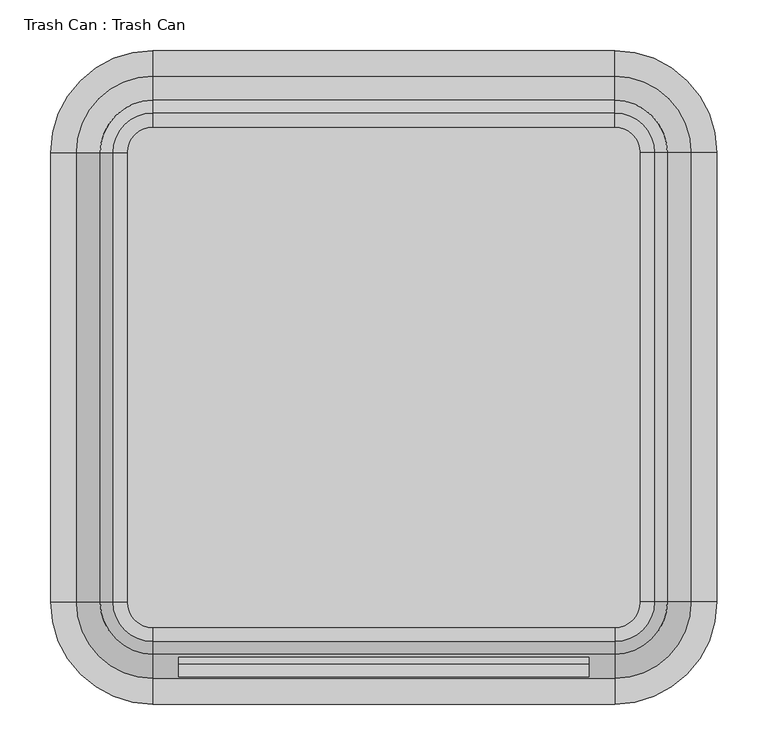
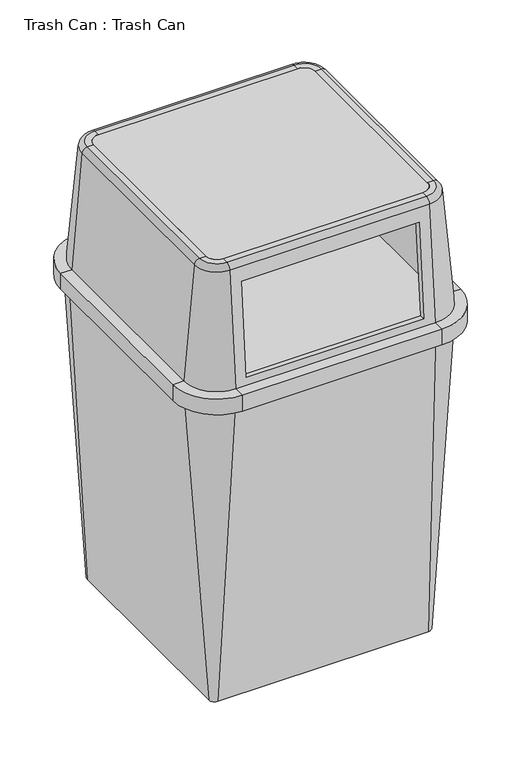
"""IFC4 building model written with IfcOpenShell, lengths in millimetres: geographic element geometry, Trash Can : Trash Can."""

from ifc_helpers import new_model, si_unit, point, frame, frame_2d, origin, place, context, project, spatial, polyline, circle_curve, ellipse_curve, trimmed, segment, composite_curve, outline, extrude, source, transform, mapped, element, save
from ifc_brep_helpers import plane_surface, cylinder_surface, revolved_surface, spline_surface, advanced_brep


def trash_can_trash_can_952d1acd(model_context):
    return source(origin(), model_context, "Body", "SolidModel", [
        advanced_brep(
        [(-254.0, 215.9, 1066.8), (-228.6, 241.3, 1066.8), (-228.6, 255.0625941, 1066.8), (-267.7625941, 215.9, 1066.8), (-254.0, 215.9, 1054.1), (-228.6, 241.3, 1054.1), (-267.7625941, 215.9, 1054.1), (-228.6, 255.0625941, 1054.1), (-292.6673476, 215.9, 769.437365), (-228.6, 279.9673476, 769.437365), (-317.0047535, 215.9, 769.437365), (-228.6, 304.3047535, 769.437365), (-317.0047535, 215.9, 744.037365), (-228.6, 304.3047535, 744.037365), (-329.7047535, 215.9, 744.037365), (-228.6, 317.0047535, 744.037365), (-329.7047535, 215.9, 782.137365), (-228.6, 317.0047535, 782.137365), (-304.3047535, 215.9, 782.137365), (-228.6, 291.6047535, 782.137365), (-280.4142668, 215.9, 1055.2068779), (-228.6, 267.7142668, 1055.2068779), (-267.7625941, -228.6, 1066.8), (-254.0, -228.6, 1066.8), (-254.0, -228.6, 1054.1), (-267.7625941, -228.6, 1054.1), (-292.6673476, -228.6, 769.437365), (-317.0047535, -228.6, 769.437365), (-317.0047535, -228.6, 744.037365), (-329.7047535, -228.6, 744.037365), (-329.7047535, -228.6, 782.137365), (-304.3047535, -228.6, 782.137365), (-280.4142668, -228.6, 1055.2068779), (-228.6, -267.7625941, 1066.8), (-228.6, -254.0, 1066.8), (-228.6, -254.0, 1054.1), (-228.6, -267.7625941, 1054.1), (-228.6, -292.6673476, 769.437365), (-228.6, -317.0047535, 769.437365), (-228.6, -317.0047535, 744.037365), (-228.6, -329.7047535, 744.037365), (-228.6, -329.7047535, 782.137365), (-228.6, -304.3047535, 782.137365), (-228.6, -280.4142668, 1055.2068779), (228.6, -267.7625941, 1066.8), (228.6, -254.0, 1066.8), (228.6, -254.0, 1054.1), (228.6, -267.7625941, 1054.1), (228.6, -292.6673476, 769.437365), (203.2, -290.0863084, 798.9387774), (203.2, -270.7170435, 1020.3304889), (-203.2, -270.7170435, 1020.3304889), (-203.2, -290.0863084, 798.9387774), (228.6, -317.0047535, 769.437365), (228.6, -317.0047535, 744.037365), (228.6, -329.7047535, 744.037365), (228.6, -329.7047535, 782.137365), (228.6, -304.3047535, 782.137365), (228.6, -280.4142668, 1055.2068779), (203.2, -283.3687161, 1021.4373669), (203.2, -302.7379811, 800.0456554), (-203.2, -302.7379811, 800.0456554), (-203.2, -283.3687161, 1021.4373669), (267.7625941, -228.6, 1066.8), (254.0, -228.6, 1066.8), (254.0, -228.6, 1054.1), (267.7625941, -228.6, 1054.1), (292.6673476, -228.6, 769.437365), (317.0047535, -228.6, 769.437365), (317.0047535, -228.6, 744.037365), (329.7047535, -228.6, 744.037365), (329.7047535, -228.6, 782.137365), (304.3047535, -228.6, 782.137365), (280.4142668, -228.6, 1055.2068779), (267.7625941, 215.9, 1066.8), (254.0, 215.9, 1066.8), (254.0, 215.9, 1054.1), (267.7625941, 215.9, 1054.1), (292.6673476, 215.9, 769.437365), (317.0047535, 215.9, 769.437365), (317.0047535, 215.9, 744.037365), (329.7047535, 215.9, 744.037365), (329.7047535, 215.9, 782.137365), (304.3047535, 215.9, 782.137365), (280.4142668, 215.9, 1055.2068779), (228.6, 255.0625941, 1066.8), (228.6, 241.3, 1066.8), (228.6, 241.3, 1054.1), (228.6, 255.0625941, 1054.1), (228.6, 279.9673476, 769.437365), (228.6, 304.3047535, 769.437365), (228.6, 304.3047535, 744.037365), (228.6, 317.0047535, 744.037365), (228.6, 317.0047535, 782.137365), (228.6, 291.6047535, 782.137365), (228.6, 267.7142668, 1055.2068779)],
        [
            (0, 1, circle_curve(frame((-228.6, 215.9, 1066.8), z_axis=(0.0, 0.0, -1.0), x_axis=(0.0, 1.0, 0.0)), 25.4)),
            (1, 2),
            (2, 3, circle_curve(frame((-228.6, 215.9, 1066.8), z_axis=(0.0, 0.0, 1.0), x_axis=(0.0, 1.0, 0.0)), 39.1625941)),
            (3, 0),
            (0, 4),
            (4, 5, circle_curve(frame((-228.6, 215.9, 1054.1), z_axis=(0.0, 0.0, -1.0), x_axis=(0.0, 1.0, 0.0)), 25.4)),
            (5, 1),
            (4, 6),
            (6, 7, circle_curve(frame((-228.6, 215.9, 1054.1), z_axis=(0.0, 0.0, -1.0), x_axis=(0.0, 1.0, 0.0)), 39.1625941)),
            (7, 5),
            (6, 8),
            (8, 9, circle_curve(frame((-228.6, 215.9, 769.437365), z_axis=(0.0, 0.0, -1.0), x_axis=(0.0, 1.0, 0.0)), 64.0673476)),
            (9, 7),
            (8, 10),
            (10, 11, circle_curve(frame((-228.6, 215.9, 769.437365), z_axis=(0.0, 0.0, -1.0), x_axis=(0.0, 1.0, 0.0)), 88.4047535)),
            (11, 9),
            (10, 12),
            (12, 13, circle_curve(frame((-228.6, 215.9, 744.037365), z_axis=(0.0, 0.0, -1.0), x_axis=(0.0, 1.0, 0.0)), 88.4047535)),
            (13, 11),
            (12, 14),
            (14, 15, circle_curve(frame((-228.6, 215.9, 744.037365), z_axis=(0.0, 0.0, -1.0), x_axis=(0.0, 1.0, 0.0)), 101.1047535)),
            (15, 13),
            (14, 16),
            (16, 17, circle_curve(frame((-228.6, 215.9, 782.137365), z_axis=(0.0, 0.0, -1.0), x_axis=(0.0, 1.0, 0.0)), 101.1047535)),
            (17, 15),
            (16, 18),
            (18, 19, circle_curve(frame((-228.6, 215.9, 782.137365), z_axis=(0.0, 0.0, -1.0), x_axis=(0.0, 1.0, 0.0)), 75.7047535)),
            (19, 17),
            (18, 20),
            (20, 21, circle_curve(frame((-228.6, 215.9, 1055.2068779), z_axis=(0.0, 0.0, -1.0), x_axis=(0.0, 1.0, 0.0)), 51.8142668)),
            (21, 19),
            (2, 21, circle_curve(frame((-228.6, 255.0625941, 1054.1), z_axis=(-1.0, 0.0, 0.0), x_axis=(0.0, -1.0, 0.0)), 12.7)),
            (20, 3, circle_curve(frame((-267.7625941, 215.9, 1054.1), z_axis=(0.0, 1.0, 0.0), x_axis=(1.0, 0.0, 0.0)), 12.7)),
            (3, 22),
            (22, 23),
            (23, 0),
            (23, 24),
            (24, 4),
            (24, 25),
            (25, 6),
            (25, 26),
            (26, 8),
            (26, 27),
            (27, 10),
            (27, 28),
            (28, 12),
            (28, 29),
            (29, 14),
            (29, 30),
            (30, 16),
            (30, 31),
            (31, 18),
            (31, 32),
            (32, 20),
            (32, 22, circle_curve(frame((-267.7625941, -228.6, 1054.1), z_axis=(0.0, 1.0, 0.0), x_axis=(1.0, 0.0, 0.0)), 12.7)),
            (22, 33, circle_curve(frame((-228.6, -228.6, 1066.8), z_axis=(0.0, 0.0, 1.0), x_axis=(-1.0, 0.0, 0.0)), 39.1625941)),
            (33, 34),
            (34, 23, circle_curve(frame((-228.6, -228.6, 1066.8), z_axis=(0.0, 0.0, -1.0), x_axis=(-1.0, 0.0, 0.0)), 25.4)),
            (34, 35),
            (35, 24, circle_curve(frame((-228.6, -228.6, 1054.1), z_axis=(0.0, 0.0, -1.0), x_axis=(-1.0, 0.0, 0.0)), 25.4)),
            (35, 36),
            (36, 25, circle_curve(frame((-228.6, -228.6, 1054.1), z_axis=(0.0, 0.0, -1.0), x_axis=(-1.0, 0.0, 0.0)), 39.1625941)),
            (36, 37),
            (37, 26, circle_curve(frame((-228.6, -228.6, 769.437365), z_axis=(0.0, 0.0, -1.0), x_axis=(-1.0, 0.0, 0.0)), 64.0673476)),
            (37, 38),
            (38, 27, circle_curve(frame((-228.6, -228.6, 769.437365), z_axis=(0.0, 0.0, -1.0), x_axis=(-1.0, 0.0, 0.0)), 88.4047535)),
            (38, 39),
            (39, 28, circle_curve(frame((-228.6, -228.6, 744.037365), z_axis=(0.0, 0.0, -1.0), x_axis=(-1.0, 0.0, 0.0)), 88.4047535)),
            (39, 40),
            (40, 29, circle_curve(frame((-228.6, -228.6, 744.037365), z_axis=(0.0, 0.0, -1.0), x_axis=(-1.0, 0.0, 0.0)), 101.1047535)),
            (40, 41),
            (41, 30, circle_curve(frame((-228.6, -228.6, 782.137365), z_axis=(0.0, 0.0, -1.0), x_axis=(-1.0, 0.0, 0.0)), 101.1047535)),
            (41, 42),
            (42, 31, circle_curve(frame((-228.6, -228.6, 782.137365), z_axis=(0.0, 0.0, -1.0), x_axis=(-1.0, 0.0, 0.0)), 75.7047535)),
            (42, 43),
            (43, 32, circle_curve(frame((-228.6, -228.6, 1055.2068779), z_axis=(0.0, 0.0, -1.0), x_axis=(-1.0, 0.0, 0.0)), 51.8142668)),
            (43, 33, circle_curve(frame((-228.6, -267.7625941, 1054.1), z_axis=(-1.0, 0.0, 0.0), x_axis=(0.0, 1.0, 0.0)), 12.7)),
            (33, 44),
            (44, 45),
            (45, 34),
            (45, 46),
            (46, 35),
            (46, 47),
            (47, 36),
            (47, 48),
            (48, 37),
            (49, 50),
            (50, 51),
            (51, 52),
            (52, 49),
            (48, 53),
            (53, 38),
            (53, 54),
            (54, 39),
            (54, 55),
            (55, 40),
            (55, 56),
            (56, 41),
            (56, 57),
            (57, 42),
            (57, 58),
            (58, 43),
            (59, 60),
            (60, 61),
            (61, 62),
            (62, 59),
            (58, 44, circle_curve(frame((228.6, -267.7625941, 1054.1), z_axis=(-1.0, 0.0, 0.0), x_axis=(0.0, 1.0, 0.0)), 12.7)),
            (44, 63, circle_curve(frame((228.6, -228.6, 1066.8), z_axis=(0.0, 0.0, 1.0), x_axis=(0.0, -1.0, 0.0)), 39.1625941)),
            (63, 64),
            (64, 45, circle_curve(frame((228.6, -228.6, 1066.8), z_axis=(0.0, 0.0, -1.0), x_axis=(0.0, -1.0, 0.0)), 25.4)),
            (64, 65),
            (65, 46, circle_curve(frame((228.6, -228.6, 1054.1), z_axis=(0.0, 0.0, -1.0), x_axis=(0.0, -1.0, 0.0)), 25.4)),
            (65, 66),
            (66, 47, circle_curve(frame((228.6, -228.6, 1054.1), z_axis=(0.0, 0.0, -1.0), x_axis=(0.0, -1.0, 0.0)), 39.1625941)),
            (66, 67),
            (67, 48, circle_curve(frame((228.6, -228.6, 769.437365), z_axis=(0.0, 0.0, -1.0), x_axis=(0.0, -1.0, 0.0)), 64.0673476)),
            (67, 68),
            (68, 53, circle_curve(frame((228.6, -228.6, 769.437365), z_axis=(0.0, 0.0, -1.0), x_axis=(0.0, -1.0, 0.0)), 88.4047535)),
            (68, 69),
            (69, 54, circle_curve(frame((228.6, -228.6, 744.037365), z_axis=(0.0, 0.0, -1.0), x_axis=(0.0, -1.0, 0.0)), 88.4047535)),
            (69, 70),
            (70, 55, circle_curve(frame((228.6, -228.6, 744.037365), z_axis=(0.0, 0.0, -1.0), x_axis=(0.0, -1.0, 0.0)), 101.1047535)),
            (70, 71),
            (71, 56, circle_curve(frame((228.6, -228.6, 782.137365), z_axis=(0.0, 0.0, -1.0), x_axis=(0.0, -1.0, 0.0)), 101.1047535)),
            (71, 72),
            (72, 57, circle_curve(frame((228.6, -228.6, 782.137365), z_axis=(0.0, 0.0, -1.0), x_axis=(0.0, -1.0, 0.0)), 75.7047535)),
            (72, 73),
            (73, 58, circle_curve(frame((228.6, -228.6, 1055.2068779), z_axis=(0.0, 0.0, -1.0), x_axis=(0.0, -1.0, 0.0)), 51.8142668)),
            (73, 63, circle_curve(frame((267.7625941, -228.6, 1054.1), z_axis=(0.0, -1.0, 0.0), x_axis=(-1.0, 0.0, 0.0)), 12.7)),
            (63, 74),
            (74, 75),
            (75, 64),
            (75, 76),
            (76, 65),
            (76, 77),
            (77, 66),
            (77, 78),
            (78, 67),
            (78, 79),
            (79, 68),
            (79, 80),
            (80, 69),
            (80, 81),
            (81, 70),
            (81, 82),
            (82, 71),
            (82, 83),
            (83, 72),
            (83, 84),
            (84, 73),
            (84, 74, circle_curve(frame((267.7625941, 215.9, 1054.1), z_axis=(0.0, -1.0, 0.0), x_axis=(-1.0, 0.0, 0.0)), 12.7)),
            (74, 85, circle_curve(frame((228.6, 215.9, 1066.8), z_axis=(0.0, 0.0, 1.0), x_axis=(1.0, 0.0, 0.0)), 39.1625941)),
            (85, 86),
            (86, 75, circle_curve(frame((228.6, 215.9, 1066.8), z_axis=(0.0, 0.0, -1.0), x_axis=(1.0, 0.0, 0.0)), 25.4)),
            (86, 87),
            (87, 76, circle_curve(frame((228.6, 215.9, 1054.1), z_axis=(0.0, 0.0, -1.0), x_axis=(1.0, 0.0, 0.0)), 25.4)),
            (87, 88),
            (88, 77, circle_curve(frame((228.6, 215.9, 1054.1), z_axis=(0.0, 0.0, -1.0), x_axis=(1.0, 0.0, 0.0)), 39.1625941)),
            (88, 89),
            (89, 78, circle_curve(frame((228.6, 215.9, 769.437365), z_axis=(0.0, 0.0, -1.0), x_axis=(1.0, 0.0, 0.0)), 64.0673476)),
            (89, 90),
            (90, 79, circle_curve(frame((228.6, 215.9, 769.437365), z_axis=(0.0, 0.0, -1.0), x_axis=(1.0, 0.0, 0.0)), 88.4047535)),
            (90, 91),
            (91, 80, circle_curve(frame((228.6, 215.9, 744.037365), z_axis=(0.0, 0.0, -1.0), x_axis=(1.0, 0.0, 0.0)), 88.4047535)),
            (91, 92),
            (92, 81, circle_curve(frame((228.6, 215.9, 744.037365), z_axis=(0.0, 0.0, -1.0), x_axis=(1.0, 0.0, 0.0)), 101.1047535)),
            (92, 93),
            (93, 82, circle_curve(frame((228.6, 215.9, 782.137365), z_axis=(0.0, 0.0, -1.0), x_axis=(1.0, 0.0, 0.0)), 101.1047535)),
            (93, 94),
            (94, 83, circle_curve(frame((228.6, 215.9, 782.137365), z_axis=(0.0, 0.0, -1.0), x_axis=(1.0, 0.0, 0.0)), 75.7047535)),
            (94, 95),
            (95, 84, circle_curve(frame((228.6, 215.9, 1055.2068779), z_axis=(0.0, 0.0, -1.0), x_axis=(1.0, 0.0, 0.0)), 51.8142668)),
            (95, 85, circle_curve(frame((228.6, 255.0625941, 1054.1), z_axis=(1.0, 0.0, 0.0), x_axis=(0.0, -1.0, 0.0)), 12.7)),
            (1, 86),
            (85, 2),
            (5, 87),
            (7, 88),
            (9, 89),
            (11, 90),
            (13, 91),
            (15, 92),
            (17, 93),
            (19, 94),
            (21, 95),
            (59, 50),
            (49, 60),
            (52, 61),
            (51, 62),
        ],
        [
            plane_surface(frame((-228.6, 215.9, 1066.8), z_axis=(0.0, 0.0, 1.0), x_axis=(0.0, 1.0, 0.0))),
            revolved_surface(polyline([(-228.6, 241.3, 1066.8), (-228.6, 241.3, 1054.1)]), (-228.6, 215.9, 0.0), (0.0, 0.0, 1.0)),
            plane_surface(frame((-228.6, 215.9, 1054.1), z_axis=(0.0, 0.0, -1.0), x_axis=(0.0, 1.0, 0.0))),
            revolved_surface(polyline([(-228.6, 255.0625941, 1054.1), (-228.6, 279.9673476, 769.437365)]), (-228.6, 215.9, 0.0), (0.0, 0.0, 1.0)),
            plane_surface(frame((-228.6, 215.9, 769.437365), z_axis=(0.0, 0.0, -1.0), x_axis=(0.0, 1.0, 0.0))),
            revolved_surface(polyline([(-228.6, 304.3047535, 769.437365), (-228.6, 304.3047535, 744.037365)]), (-228.6, 215.9, 0.0), (0.0, 0.0, 1.0)),
            plane_surface(frame((-228.6, 215.9, 744.037365), z_axis=(0.0, 0.0, -1.0), x_axis=(0.0, 1.0, 0.0))),
            cylinder_surface(frame((-228.6, 215.9, 0.0), z_axis=(0.0, 0.0, 1.0), x_axis=(0.0, 1.0, 0.0)), 101.1047535),
            plane_surface(frame((-228.6, 215.9, 782.137365), z_axis=(0.0, 0.0, 1.0), x_axis=(0.0, 1.0, 0.0))),
            revolved_surface(polyline([(-228.6, 291.6047535, 782.137365), (-228.6, 267.7142668, 1055.2068779)]), (-228.6, 215.9, 0.0), (0.0, 0.0, 1.0)),
            revolved_surface(trimmed(ellipse_curve(frame((-228.6, 255.0625941, 1054.1), z_axis=(1.0, 0.0, 0.0), x_axis=(0.0, -1.0, 0.0)), 12.7, 12.7), [point((-228.6, 267.7142668, 1055.2068779))], [point((-228.6, 255.0625941, 1066.8))], True, "CARTESIAN"), (-228.6, 215.9, 0.0), (0.0, 0.0, 1.0)),
            plane_surface(frame((-267.7625941, 215.9, 1066.8), z_axis=(0.0, 0.0, 1.0), x_axis=(0.0, -1.0, 0.0))),
            plane_surface(frame((-254.0, 215.9, 1066.8), z_axis=(1.0, 0.0, 0.0), x_axis=(0.0, -1.0, 0.0))),
            plane_surface(frame((-254.0, 215.9, 1054.1), z_axis=(0.0, 0.0, -1.0), x_axis=(0.0, -1.0, 0.0))),
            plane_surface(frame((-267.7625941, 215.9, 1054.1), z_axis=(0.9961946980917451, 0.0, -0.08715574274766279), x_axis=(0.0, -1.0, 0.0))),
            plane_surface(frame((-292.6673476, 215.9, 769.437365), z_axis=(0.0, 0.0, -1.0), x_axis=(0.0, -1.0, 0.0))),
            plane_surface(frame((-317.0047535, 215.9, 769.437365), z_axis=(1.0, 0.0, 0.0), x_axis=(0.0, -1.0, 0.0))),
            plane_surface(frame((-317.0047535, 215.9, 744.037365), z_axis=(0.0, 0.0, -1.0), x_axis=(0.0, -1.0, 0.0))),
            plane_surface(frame((-329.7047535, 215.9, 744.037365), z_axis=(-1.0, 0.0, 0.0), x_axis=(0.0, -1.0, 0.0))),
            plane_surface(frame((-329.7047535, 215.9, 782.137365), z_axis=(0.0, 0.0, 1.0), x_axis=(0.0, -1.0, 0.0))),
            plane_surface(frame((-304.3047535, 215.9, 782.137365), z_axis=(-0.9961946980917452, 0.0, 0.08715574274766147), x_axis=(0.0, -1.0, 0.0))),
            cylinder_surface(frame((-267.7625941, 215.9, 1054.1), z_axis=(0.0, 1.0, 0.0), x_axis=(1.0, 0.0, 0.0)), 12.7),
            plane_surface(frame((-228.6, -228.6, 1066.8), z_axis=(0.0, 0.0, 1.0), x_axis=(-1.0, 0.0, 0.0))),
            revolved_surface(polyline([(-254.0, -228.6, 1066.8), (-254.0, -228.6, 1054.1)]), (-228.6, -228.6, 0.0), (0.0, 0.0, 1.0)),
            plane_surface(frame((-228.6, -228.6, 1054.1), z_axis=(0.0, 0.0, -1.0), x_axis=(-1.0, 0.0, 0.0))),
            revolved_surface(polyline([(-267.7625941, -228.6, 1054.1), (-292.6673476, -228.6, 769.437365)]), (-228.6, -228.6, 0.0), (0.0, 0.0, 1.0)),
            plane_surface(frame((-228.6, -228.6, 769.437365), z_axis=(0.0, 0.0, -1.0), x_axis=(-1.0, 0.0, 0.0))),
            revolved_surface(polyline([(-317.0047535, -228.6, 769.437365), (-317.0047535, -228.6, 744.037365)]), (-228.6, -228.6, 0.0), (0.0, 0.0, 1.0)),
            plane_surface(frame((-228.6, -228.6, 744.037365), z_axis=(0.0, 0.0, -1.0), x_axis=(-1.0, 0.0, 0.0))),
            cylinder_surface(frame((-228.6, -228.6, 0.0), z_axis=(0.0, 0.0, 1.0), x_axis=(-1.0, 0.0, 0.0)), 101.1047535),
            plane_surface(frame((-228.6, -228.6, 782.137365), z_axis=(0.0, 0.0, 1.0), x_axis=(-1.0, 0.0, 0.0))),
            revolved_surface(polyline([(-304.3047535, -228.6, 782.137365), (-280.4142668, -228.6, 1055.2068779)]), (-228.6, -228.6, 0.0), (0.0, 0.0, 1.0)),
            revolved_surface(trimmed(ellipse_curve(frame((-267.7625941, -228.6, 1054.1), z_axis=(0.0, 1.0, 0.0), x_axis=(1.0, 0.0, 0.0)), 12.7, 12.7), [point((-280.4142668, -228.6, 1055.2068779))], [point((-267.7625941, -228.6, 1066.8))], True, "CARTESIAN"), (-228.6, -228.6, 0.0), (0.0, 0.0, 1.0)),
            plane_surface(frame((-228.6, -267.7625941, 1066.8), z_axis=(0.0, 0.0, 1.0), x_axis=(1.0, 0.0, 0.0))),
            plane_surface(frame((-228.6, -254.0, 1066.8), z_axis=(0.0, 1.0, 0.0), x_axis=(1.0, 0.0, 0.0))),
            plane_surface(frame((-228.6, -254.0, 1054.1), z_axis=(0.0, 0.0, -1.0), x_axis=(1.0, 0.0, 0.0))),
            plane_surface(frame((-228.6, -267.7625941, 1054.1), z_axis=(0.0, 0.9961946980917451, -0.08715574274766279), x_axis=(1.0, 0.0, 0.0))),
            plane_surface(frame((-228.6, -292.6673476, 769.437365), z_axis=(0.0, 0.0, -1.0), x_axis=(1.0, 0.0, 0.0))),
            plane_surface(frame((-228.6, -317.0047535, 769.437365), z_axis=(0.0, 1.0, 0.0), x_axis=(1.0, 0.0, 0.0))),
            plane_surface(frame((-228.6, -317.0047535, 744.037365), z_axis=(0.0, 0.0, -1.0), x_axis=(1.0, 0.0, 0.0))),
            plane_surface(frame((-228.6, -329.7047535, 744.037365), z_axis=(0.0, -1.0, 0.0), x_axis=(1.0, 0.0, 0.0))),
            plane_surface(frame((-228.6, -329.7047535, 782.137365), z_axis=(0.0, 0.0, 1.0), x_axis=(1.0, 0.0, 0.0))),
            plane_surface(frame((-228.6, -304.3047535, 782.137365), z_axis=(0.0, -0.9961946980917452, 0.08715574274766147), x_axis=(1.0, 0.0, 0.0))),
            cylinder_surface(frame((-228.6, -267.7625941, 1054.1), z_axis=(-1.0, 0.0, 0.0), x_axis=(0.0, 1.0, 0.0)), 12.7),
            plane_surface(frame((228.6, -228.6, 1066.8), z_axis=(0.0, 0.0, 1.0), x_axis=(0.0, -1.0, 0.0))),
            revolved_surface(polyline([(228.6, -254.0, 1066.8), (228.6, -254.0, 1054.1)]), (228.6, -228.6, 0.0), (0.0, 0.0, 1.0)),
            plane_surface(frame((228.6, -228.6, 1054.1), z_axis=(0.0, 0.0, -1.0), x_axis=(0.0, -1.0, 0.0))),
            revolved_surface(polyline([(228.6, -267.7625941, 1054.1), (228.6, -292.6673476, 769.437365)]), (228.6, -228.6, 0.0), (0.0, 0.0, 1.0)),
            plane_surface(frame((228.6, -228.6, 769.437365), z_axis=(0.0, 0.0, -1.0), x_axis=(0.0, -1.0, 0.0))),
            revolved_surface(polyline([(228.6, -317.0047535, 769.437365), (228.6, -317.0047535, 744.037365)]), (228.6, -228.6, 0.0), (0.0, 0.0, 1.0)),
            plane_surface(frame((228.6, -228.6, 744.037365), z_axis=(0.0, 0.0, -1.0), x_axis=(0.0, -1.0, 0.0))),
            cylinder_surface(frame((228.6, -228.6, 0.0), z_axis=(0.0, 0.0, 1.0), x_axis=(0.0, -1.0, 0.0)), 101.1047535),
            plane_surface(frame((228.6, -228.6, 782.137365), z_axis=(0.0, 0.0, 1.0), x_axis=(0.0, -1.0, 0.0))),
            revolved_surface(polyline([(228.6, -304.3047535, 782.137365), (228.6, -280.4142668, 1055.2068779)]), (228.6, -228.6, 0.0), (0.0, 0.0, 1.0)),
            revolved_surface(trimmed(ellipse_curve(frame((228.6, -267.7625941, 1054.1), z_axis=(-1.0, 0.0, 0.0), x_axis=(0.0, 1.0, 0.0)), 12.7, 12.7), [point((228.6, -280.4142668, 1055.2068779))], [point((228.6, -267.7625941, 1066.8))], True, "CARTESIAN"), (228.6, -228.6, 0.0), (0.0, 0.0, 1.0)),
            plane_surface(frame((267.7625941, -228.6, 1066.8), z_axis=(0.0, 0.0, 1.0), x_axis=(0.0, 1.0, 0.0))),
            plane_surface(frame((254.0, -228.6, 1066.8), z_axis=(-1.0, 0.0, 0.0), x_axis=(0.0, 1.0, 0.0))),
            plane_surface(frame((254.0, -228.6, 1054.1), z_axis=(0.0, 0.0, -1.0), x_axis=(0.0, 1.0, 0.0))),
            plane_surface(frame((267.7625941, -228.6, 1054.1), z_axis=(-0.9961946980917451, 0.0, -0.08715574274766279), x_axis=(0.0, 1.0, 0.0))),
            plane_surface(frame((292.6673476, -228.6, 769.437365), z_axis=(0.0, 0.0, -1.0), x_axis=(0.0, 1.0, 0.0))),
            plane_surface(frame((317.0047535, -228.6, 769.437365), z_axis=(-1.0, 0.0, 0.0), x_axis=(0.0, 1.0, 0.0))),
            plane_surface(frame((317.0047535, -228.6, 744.037365), z_axis=(0.0, 0.0, -1.0), x_axis=(0.0, 1.0, 0.0))),
            plane_surface(frame((329.7047535, -228.6, 744.037365), z_axis=(1.0, 0.0, 0.0), x_axis=(0.0, 1.0, 0.0))),
            plane_surface(frame((329.7047535, -228.6, 782.137365), z_axis=(0.0, 0.0, 1.0), x_axis=(0.0, 1.0, 0.0))),
            plane_surface(frame((304.3047535, -228.6, 782.137365), z_axis=(0.9961946980917452, 0.0, 0.08715574274766147), x_axis=(0.0, 1.0, 0.0))),
            cylinder_surface(frame((267.7625941, -228.6, 1054.1), z_axis=(0.0, -1.0, 0.0), x_axis=(-1.0, 0.0, 0.0)), 12.7),
            plane_surface(frame((228.6, 215.9, 1066.8), z_axis=(0.0, 0.0, 1.0), x_axis=(1.0, 0.0, 0.0))),
            revolved_surface(polyline([(254.0, 215.9, 1066.8), (254.0, 215.9, 1054.1)]), (228.6, 215.9, 0.0), (0.0, 0.0, 1.0)),
            plane_surface(frame((228.6, 215.9, 1054.1), z_axis=(0.0, 0.0, -1.0), x_axis=(1.0, 0.0, 0.0))),
            revolved_surface(polyline([(267.7625941, 215.9, 1054.1), (292.6673476, 215.9, 769.437365)]), (228.6, 215.9, 0.0), (0.0, 0.0, 1.0)),
            plane_surface(frame((228.6, 215.9, 769.437365), z_axis=(0.0, 0.0, -1.0), x_axis=(1.0, 0.0, 0.0))),
            revolved_surface(polyline([(317.0047535, 215.9, 769.437365), (317.0047535, 215.9, 744.037365)]), (228.6, 215.9, 0.0), (0.0, 0.0, 1.0)),
            plane_surface(frame((228.6, 215.9, 744.037365), z_axis=(0.0, 0.0, -1.0), x_axis=(1.0, 0.0, 0.0))),
            cylinder_surface(frame((228.6, 215.9, 0.0), z_axis=(0.0, 0.0, 1.0), x_axis=(1.0, 0.0, 0.0)), 101.1047535),
            plane_surface(frame((228.6, 215.9, 782.137365), z_axis=(0.0, 0.0, 1.0), x_axis=(1.0, 0.0, 0.0))),
            revolved_surface(polyline([(304.3047535, 215.9, 782.137365), (280.4142668, 215.9, 1055.2068779)]), (228.6, 215.9, 0.0), (0.0, 0.0, 1.0)),
            revolved_surface(trimmed(ellipse_curve(frame((267.7625941, 215.9, 1054.1), z_axis=(0.0, -1.0, 0.0), x_axis=(-1.0, 0.0, 0.0)), 12.7, 12.7), [point((280.4142668, 215.9, 1055.2068779))], [point((267.7625941, 215.9, 1066.8))], True, "CARTESIAN"), (228.6, 215.9, 0.0), (0.0, 0.0, 1.0)),
            plane_surface(frame((228.6, 255.0625941, 1066.8), z_axis=(0.0, 0.0, 1.0), x_axis=(-1.0, 0.0, 0.0))),
            plane_surface(frame((228.6, 241.3, 1066.8), z_axis=(0.0, -1.0, 0.0), x_axis=(-1.0, 0.0, 0.0))),
            plane_surface(frame((228.6, 241.3, 1054.1), z_axis=(0.0, 0.0, -1.0), x_axis=(-1.0, 0.0, 0.0))),
            plane_surface(frame((228.6, 255.0625941, 1054.1), z_axis=(0.0, -0.9961946980917451, -0.08715574274766279), x_axis=(-1.0, 0.0, 0.0))),
            plane_surface(frame((228.6, 279.9673476, 769.437365), z_axis=(0.0, 0.0, -1.0), x_axis=(-1.0, 0.0, 0.0))),
            plane_surface(frame((228.6, 304.3047535, 769.437365), z_axis=(0.0, -1.0, 0.0), x_axis=(-1.0, 0.0, 0.0))),
            plane_surface(frame((228.6, 304.3047535, 744.037365), z_axis=(0.0, 0.0, -1.0), x_axis=(-1.0, 0.0, 0.0))),
            plane_surface(frame((228.6, 317.0047535, 744.037365), z_axis=(0.0, 1.0, 0.0), x_axis=(-1.0, 0.0, 0.0))),
            plane_surface(frame((228.6, 317.0047535, 782.137365), z_axis=(0.0, 0.0, 1.0), x_axis=(-1.0, 0.0, 0.0))),
            plane_surface(frame((228.6, 291.6047535, 782.137365), z_axis=(0.0, 0.9961946980917452, 0.08715574274766147), x_axis=(-1.0, 0.0, 0.0))),
            cylinder_surface(frame((228.6, 255.0625941, 1054.1), z_axis=(1.0, 0.0, 0.0), x_axis=(0.0, -1.0, 0.0)), 12.7),
            plane_surface(frame((203.2, -213.4252032, 1015.3181024), z_axis=(-1.0, 0.0, 0.0), x_axis=(0.0, -0.9961946980917452, 0.08715574274766175))),
            plane_surface(frame((203.2, -232.7944681, 793.9263909), z_axis=(0.0, 0.08715574274766175, 0.9961946980917452), x_axis=(0.0, -0.9961946980917452, 0.08715574274766175))),
            plane_surface(frame((-203.2, -232.7944681, 793.9263909), z_axis=(1.0, 0.0, 0.0), x_axis=(0.0, -0.9961946980917452, 0.08715574274766175))),
            plane_surface(frame((-203.2, -213.4252032, 1015.3181024), z_axis=(0.0, -0.08715574274766175, -0.9961946980917452), x_axis=(0.0, -0.9961946980917452, 0.08715574274766175))),
        ],
        [
            (0, [[1, 2, 3, 4]]),
            (1, [[-1, 5, 6, 7]]),
            (2, [[-6, 8, 9, 10]]),
            (3, [[-9, 11, 12, 13]]),
            (4, [[-12, 14, 15, 16]]),
            (5, [[-15, 17, 18, 19]]),
            (6, [[-18, 20, 21, 22]]),
            (7, [[-21, 23, 24, 25]]),
            (8, [[-24, 26, 27, 28]]),
            (9, [[-27, 29, 30, 31]]),
            (10, [[-3, 32, -30, 33]]),
            (11, [[-4, 34, 35, 36]]),
            (12, [[-5, -36, 37, 38]]),
            (13, [[-8, -38, 39, 40]]),
            (14, [[-11, -40, 41, 42]]),
            (15, [[-14, -42, 43, 44]]),
            (16, [[-17, -44, 45, 46]]),
            (17, [[-20, -46, 47, 48]]),
            (18, [[-23, -48, 49, 50]]),
            (19, [[-26, -50, 51, 52]]),
            (20, [[-29, -52, 53, 54]]),
            (21, [[-33, -54, 55, -34]]),
            (22, [[-35, 56, 57, 58]]),
            (23, [[-37, -58, 59, 60]]),
            (24, [[-39, -60, 61, 62]]),
            (25, [[-41, -62, 63, 64]]),
            (26, [[-43, -64, 65, 66]]),
            (27, [[-45, -66, 67, 68]]),
            (28, [[-47, -68, 69, 70]]),
            (29, [[-49, -70, 71, 72]]),
            (30, [[-51, -72, 73, 74]]),
            (31, [[-53, -74, 75, 76]]),
            (32, [[-55, -76, 77, -56]]),
            (33, [[-57, 78, 79, 80]]),
            (34, [[-59, -80, 81, 82]]),
            (35, [[-61, -82, 83, 84]]),
            (36, [[-63, -84, 85, 86], [87, 88, 89, 90]]),
            (37, [[-65, -86, 91, 92]]),
            (38, [[-67, -92, 93, 94]]),
            (39, [[-69, -94, 95, 96]]),
            (40, [[-71, -96, 97, 98]]),
            (41, [[-73, -98, 99, 100]]),
            (42, [[-75, -100, 101, 102], [103, 104, 105, 106]]),
            (43, [[-77, -102, 107, -78]]),
            (44, [[-79, 108, 109, 110]]),
            (45, [[-81, -110, 111, 112]]),
            (46, [[-83, -112, 113, 114]]),
            (47, [[-85, -114, 115, 116]]),
            (48, [[-91, -116, 117, 118]]),
            (49, [[-93, -118, 119, 120]]),
            (50, [[-95, -120, 121, 122]]),
            (51, [[-97, -122, 123, 124]]),
            (52, [[-99, -124, 125, 126]]),
            (53, [[-101, -126, 127, 128]]),
            (54, [[-107, -128, 129, -108]]),
            (55, [[-109, 130, 131, 132]]),
            (56, [[-111, -132, 133, 134]]),
            (57, [[-113, -134, 135, 136]]),
            (58, [[-115, -136, 137, 138]]),
            (59, [[-117, -138, 139, 140]]),
            (60, [[-119, -140, 141, 142]]),
            (61, [[-121, -142, 143, 144]]),
            (62, [[-123, -144, 145, 146]]),
            (63, [[-125, -146, 147, 148]]),
            (64, [[-127, -148, 149, 150]]),
            (65, [[-129, -150, 151, -130]]),
            (66, [[-131, 152, 153, 154]]),
            (67, [[-133, -154, 155, 156]]),
            (68, [[-135, -156, 157, 158]]),
            (69, [[-137, -158, 159, 160]]),
            (70, [[-139, -160, 161, 162]]),
            (71, [[-141, -162, 163, 164]]),
            (72, [[-143, -164, 165, 166]]),
            (73, [[-145, -166, 167, 168]]),
            (74, [[-147, -168, 169, 170]]),
            (75, [[-149, -170, 171, 172]]),
            (76, [[-151, -172, 173, -152]]),
            (77, [[-2, 174, -153, 175]]),
            (78, [[-7, 176, -155, -174]]),
            (79, [[-10, 177, -157, -176]]),
            (80, [[-13, 178, -159, -177]]),
            (81, [[-16, 179, -161, -178]]),
            (82, [[-19, 180, -163, -179]]),
            (83, [[-22, 181, -165, -180]]),
            (84, [[-25, 182, -167, -181]]),
            (85, [[-28, 183, -169, -182]]),
            (86, [[-31, 184, -171, -183]]),
            (87, [[-32, -175, -173, -184]]),
            (88, [[185, -87, 186, -103]]),
            (89, [[-186, -90, 187, -104]]),
            (90, [[-187, -89, 188, -105]]),
            (91, [[-185, -106, -188, -88]]),
        ],
    ),
        extrude(outline(composite_curve([segment(trimmed(circle_curve(frame_2d((241.3, 228.6)), 12.7), [point((241.3, 241.3))], [point((254.0, 228.6))], False, "CARTESIAN"), True, "CONTINUOUS"), segment(polyline([(254.0, 228.6), (254.0, -228.6)]), True, "CONTINUOUS"), segment(trimmed(circle_curve(frame_2d((228.6, -228.6)), 25.4), [point((254.0, -228.6))], [point((228.6, -254.0))], False, "CARTESIAN"), True, "CONTINUOUS"), segment(polyline([(228.6, -254.0), (-228.6, -254.0)]), True, "CONTINUOUS"), segment(trimmed(circle_curve(frame_2d((-228.6, -228.6)), 25.4), [point((-228.6, -254.0))], [point((-254.0, -228.6))], False, "CARTESIAN"), True, "CONTINUOUS"), segment(polyline([(-254.0, -228.6), (-254.0, 215.9)]), True, "CONTINUOUS"), segment(trimmed(circle_curve(frame_2d((-228.6, 215.9)), 25.4), [point((-254.0, 215.9))], [point((-228.6, 241.3))], False, "CARTESIAN"), True, "CONTINUOUS"), segment(polyline([(-228.6, 241.3), (241.3, 241.3)]), True, "CONTINUOUS")], self_intersect=False)), frame((0.0, 0.0, 1054.1), z_axis=(0.0, 0.0, 1.0), x_axis=(1.0, 0.0, 0.0)), (0.0, 0.0, 1.0), 12.7),
        advanced_brep(
        [(228.6, 304.8, 762.0), (-228.6, 304.8, 762.0), (-304.8, 228.6, 762.0), (-304.8, -228.6, 762.0), (-228.6, -304.8, 762.0), (228.6, -304.8, 762.0), (304.8, -228.6, 762.0), (304.8, 228.6, 762.0), (241.3, 254.0, 0.0), (254.0, 241.3, 0.0), (254.0, -241.3, 0.0), (241.3, -254.0, 0.0), (-241.3, -254.0, 0.0), (-254.0, -241.3, 0.0), (-254.0, 241.3, 0.0), (-241.3, 254.0, 0.0)],
        [
            (0, 1),
            (1, 2, circle_curve(frame((-228.6, 228.6, 762.0), z_axis=(0.0, 0.0, 1.0), x_axis=(1.0, 0.0, 0.0)), 76.2)),
            (2, 3),
            (3, 4, circle_curve(frame((-228.6, -228.6, 762.0), z_axis=(0.0, 0.0, 1.0), x_axis=(1.0, 0.0, 0.0)), 76.2)),
            (4, 5),
            (5, 6, circle_curve(frame((228.6, -228.6, 762.0), z_axis=(0.0, 0.0, 1.0), x_axis=(1.0, 0.0, 0.0)), 76.2)),
            (6, 7),
            (7, 0, circle_curve(frame((228.6, 228.6, 762.0), z_axis=(0.0, 0.0, 1.0), x_axis=(1.0, 0.0, 0.0)), 76.2)),
            (8, 9, circle_curve(frame((241.3, 241.3, 0.0), z_axis=(0.0, 0.0, -1.0), x_axis=(1.0, 0.0, 0.0)), 12.7)),
            (9, 10),
            (10, 11, circle_curve(frame((241.3, -241.3, 0.0), z_axis=(0.0, 0.0, -1.0), x_axis=(1.0, 0.0, 0.0)), 12.7)),
            (11, 12),
            (12, 13, circle_curve(frame((-241.3, -241.3, 0.0), z_axis=(0.0, 0.0, -1.0), x_axis=(1.0, 0.0, 0.0)), 12.7)),
            (13, 14),
            (14, 15, circle_curve(frame((-241.3, 241.3, 0.0), z_axis=(0.0, 0.0, -1.0), x_axis=(1.0, 0.0, 0.0)), 12.7)),
            (15, 8),
            (15, 1),
            (0, 8),
            (14, 2),
            (13, 3),
            (12, 4),
            (11, 5),
            (10, 6),
            (9, 7),
        ],
        [
            plane_surface(frame((0.0, 0.0, 762.0), z_axis=(0.0, 0.0, 1.0), x_axis=(-1.0, 0.0, 0.0))),
            plane_surface(frame((0.0, 0.0, 0.0), z_axis=(0.0, 0.0, -1.0), x_axis=(-1.0, 0.0, 0.0))),
            plane_surface(frame((0.0, 254.0, 0.0), z_axis=(0.0, 0.9977851578566089, -0.0665190105237736), x_axis=(-1.0, 0.0, 0.0))),
            spline_surface(2, 1, [[(-241.3, 254.0, 0.0), (-228.6, 304.8, 762.0)], [(-254.0, 254.0, 0.0), (-304.8, 304.8, 762.0)], [(-254.0, 241.3, 0.0), (-304.8, 228.6, 762.0)]], [3, 3], [2, 2], [0.0, 1.0], [0.0, 1.0], weights=[[1.0, 1.0], [0.7071067811865476, 0.7071067811865476], [1.0, 1.0]]),
            plane_surface(frame((-254.0, 0.0, 0.0), z_axis=(-0.9977851578566089, 0.0, -0.06651901052377489), x_axis=(0.0, -1.0, 0.0))),
            spline_surface(2, 1, [[(-254.0, -241.3, 0.0), (-304.8, -228.6, 762.0)], [(-254.0, -254.0, 0.0), (-304.8, -304.8, 762.0)], [(-241.3, -254.0, 0.0), (-228.6, -304.8, 762.0)]], [3, 3], [2, 2], [0.0, 1.0], [0.0, 1.0], weights=[[1.0, 1.0], [0.7071067811865476, 0.7071067811865476], [1.0, 1.0]]),
            plane_surface(frame((0.0, -254.0, 0.0), z_axis=(0.0, -0.9977851578566089, -0.06651901052377414), x_axis=(1.0, 0.0, 0.0))),
            spline_surface(2, 1, [[(241.3, -254.0, 0.0), (228.6, -304.8, 762.0)], [(254.0, -254.0, 0.0), (304.8, -304.8, 762.0)], [(254.0, -241.3, 0.0), (304.8, -228.6, 762.0)]], [3, 3], [2, 2], [0.0, 1.0], [0.0, 1.0], weights=[[1.0, 1.0], [0.7071067811865476, 0.7071067811865476], [1.0, 1.0]]),
            plane_surface(frame((254.0, 0.0, 0.0), z_axis=(0.9977851578566089, 0.0, -0.0665190105237748), x_axis=(0.0, 1.0, 0.0))),
            spline_surface(2, 1, [[(254.0, 241.3, 0.0), (304.8, 228.6, 762.0)], [(254.0, 254.0, 0.0), (304.8, 304.8, 762.0)], [(241.3, 254.0, 0.0), (228.6, 304.8, 762.0)]], [3, 3], [2, 2], [0.0, 1.0], [0.0, 1.0], weights=[[1.0, 1.0], [0.7071067811865476, 0.7071067811865476], [1.0, 1.0]]),
        ],
        [
            (0, [[1, 2, 3, 4, 5, 6, 7, 8]]),
            (1, [[9, 10, 11, 12, 13, 14, 15, 16]]),
            (2, [[-16, 17, -1, 18]]),
            (3, [[-15, 19, -2, -17]]),
            (4, [[-14, 20, -3, -19]]),
            (5, [[-13, 21, -4, -20]]),
            (6, [[-12, 22, -5, -21]]),
            (7, [[-11, 23, -6, -22]]),
            (8, [[-10, 24, -7, -23]]),
            (9, [[-9, -18, -8, -24]]),
        ],
    ),
    ])


if __name__ == "__main__":
    model = new_model("IFC4")
    model_context = context("Model", 3, world=origin())
    ifc_project = project(units=[si_unit("LENGTHUNIT", "METRE", prefix="MILLI")], contexts=[model_context])
    site = spatial("IfcSite", under=ifc_project)
    building = spatial("IfcBuilding", under=site)
    placement = place(None, origin())
    trash_can_trash_can_shape = trash_can_trash_can_952d1acd(model_context)
    element("IfcGeographicElement", 1, ObjectType="Trash Can : Trash Can", at=placement, inside=building, context=model_context, shape_type="MappedRepresentation", body=[
        mapped(trash_can_trash_can_shape, transform((0.0, 0.0, 0.0), x_axis=(1.0, 0.0, 0.0), y_axis=(0.0, 1.0, 0.0), z_axis=(0.0, 0.0, 1.0))),
    ])
    save(model, "model.ifc")

# Revit data of these elements
# Type "Trash Can : Trash Can"
#   Assembly Code = "G2040900"
# Element 1 (IfcGeographicElement, "Trash Can : Trash Can")
#   Materials on its faces: "Plastic - Gray, Dark", "Plastic, Opaque Black"
# Materials
#   "Plastic - Gray, Dark": class "Plastic", colour RGB 134 134 134, transparency 0
#   "Plastic, Opaque Black": class "Plastic", colour RGB 0 0 0, transparency 0.7, Description = "Plastic, generic, opaque black", Cost = 0
